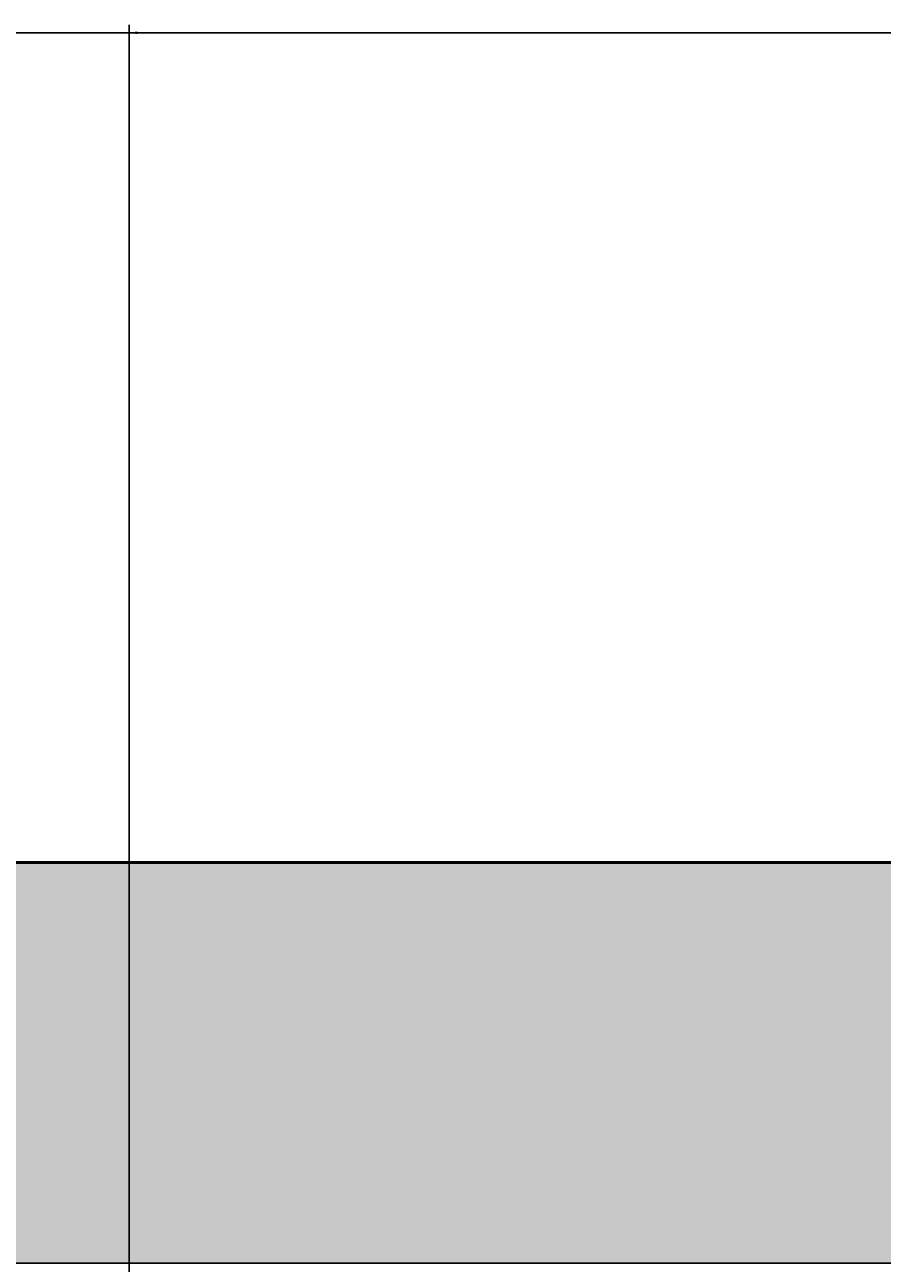
# Model space of a CAD drawing. Units: inches. Extents: x 2231 to 2461, y 2045 to 2455.
# Tile 87 of 95: x 2346 to 2365, y 2427 to 2455. Entities that reach past the tile are written whole.
import ezdxf

# ---------------------------------------------------------------- set-up
doc = ezdxf.new("R2010")
doc.units = ezdxf.units.IN
doc.layers.add('A-ANNO-DIMS', color=2, linetype='Continuous', lineweight=18)
doc.layers.add('A-WALL', color=7, linetype='Continuous', lineweight=50)
doc.layers.add('A-WALL-PATT', color=18, linetype='Continuous', lineweight=13, true_color=0x000000)
doc.styles.get("Standard").update_dxf_attribs({"font": 'arial.ttf'})
doc.dimstyles.get("Standard").update_dxf_attribs({"dimtxt": 0.18, "dimasz": 0.18, "dimexe": 0.18, "dimexo": 0.0625, "dimgap": 0.09, "dimtad": 0, "dimtih": 1, "dimtoh": 1, "dimdec": 4, "dimzin": 0, "dimdsep": 46, "dimtxsty": 'Standard', "dimcen": 0.09, "dimadec": 0, "dimazin": 0, "dimtfac": 1, "dimtdec": 4, "dimtofl": 0, "dimtmove": 0, "dimatfit": 3, "dimfxl": 1, "dimtolj": 1, "dimtzin": 0, "dimarcsym": 0})

# ---------------------------------------------------------------- blocks, each defined once
blk = doc.blocks.new('*D35')
at = {"layer": 'A-ANNO-DIMS', "color": 0, "lineweight": -2, "transparency": 16777216}
for p, q in [((2258.794, 2426.895), (2258.794, 2454.645)), ((2258.974, 2454.465), (2313.513, 2454.465)), ((2368.614, 2454.465), (2314.074, 2454.465)), ((2368.794, 2426.895), (2368.794, 2454.645))]:
    blk.add_line(p, q, dxfattribs=at)
at = {"layer": 'A-ANNO-DIMS', "color": 0, "transparency": 16777216}
for points in [[(2258.974, 2454.495), (2258.974, 2454.435), (2258.794, 2454.465)], [(2368.614, 2454.495), (2368.614, 2454.435), (2368.794, 2454.465)]]:
    blk.add_solid(points, dxfattribs=at)
at = {"layer": 'Defpoints', "color": 0, "transparency": 16777216}
for p in [(2368.794, 2454.465), (2258.794, 2426.833), (2368.794, 2426.833)]:
    blk.add_point(p, dxfattribs=at)
at = {"layer": 'A-ANNO-DIMS', "color": 0, "transparency": 16777216, "insert": (2313.794, 2454.465), "char_height": 0.18, "attachment_point": 5}
blk.add_mtext('\\A1;110', dxfattribs=at)
blk = doc.blocks.new('*D66')
at = {"layer": 'A-ANNO-DIMS', "color": 0, "lineweight": -2, "transparency": 16777216}
for p, q in [((2348.189, 2096.895), (2348.189, 2454.645)), ((2348.369, 2454.465), (2378.167, 2454.465)), ((2408.614, 2454.465), (2378.815, 2454.465)), ((2408.794, 2096.895), (2408.794, 2454.645))]:
    blk.add_line(p, q, dxfattribs=at)
at = {"layer": 'A-ANNO-DIMS', "color": 0, "transparency": 16777216}
for points in [[(2348.369, 2454.495), (2348.369, 2454.435), (2348.189, 2454.465)], [(2408.614, 2454.495), (2408.614, 2454.435), (2408.794, 2454.465)]]:
    blk.add_solid(points, dxfattribs=at)
at = {"layer": 'Defpoints', "color": 0, "transparency": 16777216}
for p in [(2408.794, 2454.465), (2348.189, 2096.833), (2408.794, 2096.833)]:
    blk.add_point(p, dxfattribs=at)
at = {"layer": 'A-ANNO-DIMS', "color": 0, "transparency": 16777216, "insert": (2378.491, 2454.465), "char_height": 0.18, "attachment_point": 5}
blk.add_mtext('\\A1;60.6', dxfattribs=at)
blk = doc.blocks.new('*D68')
at = {"layer": 'A-ANNO-DIMS', "color": 0, "lineweight": -2, "transparency": 16777216}
for p, q in [((2285.882, 2426.833), (2460.606, 2426.833)), ((2460.426, 2426.653), (2460.426, 2420.225)), ((2460.426, 2413.433), (2460.426, 2419.861)), ((2278.251, 2413.253), (2460.606, 2413.253))]:
    blk.add_line(p, q, dxfattribs=at)
at = {"layer": 'A-ANNO-DIMS', "color": 0, "transparency": 16777216}
for points in [[(2460.396, 2426.653), (2460.456, 2426.653), (2460.426, 2426.833)], [(2460.396, 2413.433), (2460.456, 2413.433), (2460.426, 2413.253)]]:
    blk.add_solid(points, dxfattribs=at)
at = {"layer": 'Defpoints', "color": 0, "transparency": 16777216}
for p in [(2285.82, 2426.833), (2460.426, 2426.833), (2278.188, 2413.253)]:
    blk.add_point(p, dxfattribs=at)
at = {"layer": 'A-ANNO-DIMS', "color": 0, "transparency": 16777216, "insert": (2460.426, 2420.043), "char_height": 0.18, "attachment_point": 5}
blk.add_mtext('\\A1;13.58', dxfattribs=at)

msp = doc.modelspace()

# ---------------------------------------------------------------- hatches: boundary and pattern name
at = {"layer": 'A-WALL-PATT'}
h = msp.add_hatch(color=256, dxfattribs=at)
h.dxf.hatch_style = 1
h.paths.add_polyline_path([(2441.7935, 2269.1535), (2432.7935, 2269.1535), (2432.7935, 2186.8328), (2396.7935, 2186.8328), (2396.7935, 2286.8328), (2394.7935, 2286.8328), (2394.7935, 2186.8328), (2334.7935, 2186.8328), (2334.7935, 2182.8328), (2432.7935, 2182.8328), (2432.7935, 2072.8328), (2416.6639, 2072.8328), (2416.6639, 2063.8328), (2441.7935, 2063.8328)])
h.paths.add_polyline_path([(2368.6639, 2072.8328), (2367.04, 2072.8328), (2330.7942, 2072.8328), (2330.7397, 2063.8328), (2368.6639, 2063.8328)])
h.paths.add_polyline_path([(2300.7392, 2068.3328), (2300.7392, 2072.8328), (2298.7935, 2072.8328), (2294.7935, 2072.8328), (2258.7935, 2072.8328), (2258.7935, 2120.8328), (2294.7935, 2120.8328), (2298.7935, 2120.8328), (2298.7935, 2128.8328), (2294.7935, 2128.8328), (2294.7935, 2124.8328), (2258.7935, 2124.8328), (2258.7935, 2182.8328), (2294.7935, 2182.8328), (2294.7935, 2174.8328), (2298.7935, 2174.8328), (2298.7935, 2182.8328), (2304.7935, 2182.8328), (2304.7935, 2186.8328), (2258.7935, 2186.8328), (2258.7935, 2221.999), (2249.7935, 2221.999), (2249.7935, 2063.8328), (2300.7392, 2063.8328)])
h.paths.add_polyline_path([(2391.9338, 2435.8328), (2333.82, 2435.8328), (2333.82, 2426.8328), (2368.7935, 2426.8328), (2368.7935, 2374.9508), (2368.7935, 2370.8328), (2372.3935, 2370.8328), (2372.7935, 2370.8328), (2372.7935, 2426.8328), (2391.9338, 2426.8328)])
h.paths.add_polyline_path([(2441.7935, 2435.8328), (2415.9338, 2435.8328), (2415.9338, 2426.8328), (2432.7935, 2426.8328), (2432.7935, 2334.8328), (2372.7935, 2334.8328), (2372.7935, 2346.8328), (2368.7935, 2346.8328), (2368.7935, 2306.8328), (2360.7935, 2306.8328), (2360.7935, 2302.8328), (2368.7935, 2302.8328), (2372.7935, 2302.8328), (2372.7935, 2330.8328), (2432.7935, 2330.8328), (2432.7935, 2317.1535), (2441.7935, 2317.1535)])
h.paths.add_polyline_path([(2285.82, 2435.8328), (2249.7935, 2435.8328), (2249.7935, 2269.999), (2258.7935, 2269.999), (2258.7935, 2302.8328), (2318.8168, 2302.8328), (2330.7935, 2302.8328), (2330.7935, 2306.8328), (2258.7935, 2306.8328), (2258.7935, 2426.8328), (2285.82, 2426.8328)])

# ---------------------------------------------------------------- linework, layer by layer
at = {"layer": 'A-WALL'}
msp.add_lwpolyline([(2300.7392, 2063.8328), (2249.7935, 2063.8328), (2249.7935, 2435.8328), (2441.7935, 2435.8328), (2441.7935, 2063.8328), (2330.7397, 2063.8328)], dxfattribs=at)

# ---------------------------------------------------------------- dimensions: what is measured, and where the dimension line sits
at = {"layer": 'A-ANNO-DIMS'}
for base, p1, p2, override, picture, middle in [((2368.7935, 2454.4653), (2258.7935, 2426.8328), (2368.7935, 2426.8328), {"dimdec": 0, "dimlfac": 1, "dimrnd": 0, "dimzin": 0, "dimdsep": 46, "dimlunit": 2}, '*D35', (2313.7935, 2454.4653)), ((2408.7935, 2454.4653), (2348.1888, 2096.8328), (2408.7935, 2096.8328), {"dimdec": 1, "dimlfac": 1, "dimrnd": 0, "dimzin": 0, "dimdsep": 46, "dimlunit": 2}, '*D66', (2378.4912, 2454.4653))]:
    dim = msp.add_linear_dim(base=base, p1=p1, p2=p2, dimstyle='Standard', override=override, dxfattribs=at)
    dim.commit()
    dim.dimension.update_dxf_attribs({"geometry": picture, "text_midpoint": middle})
dim = msp.add_linear_dim(base=(2460.426, 2426.8328), p1=(2278.1881, 2413.2534), p2=(2285.82, 2426.8328), angle=90, dimstyle='Standard', override={"dimdec": 2, "dimlfac": 1, "dimrnd": 0, "dimzin": 0, "dimdsep": 46, "dimlunit": 2}, dxfattribs=at)
dim.commit()
dim.dimension.update_dxf_attribs({"geometry": '*D68', "text_midpoint": (2460.426, 2420.0431)})

doc.saveas('drawing.dxf')
